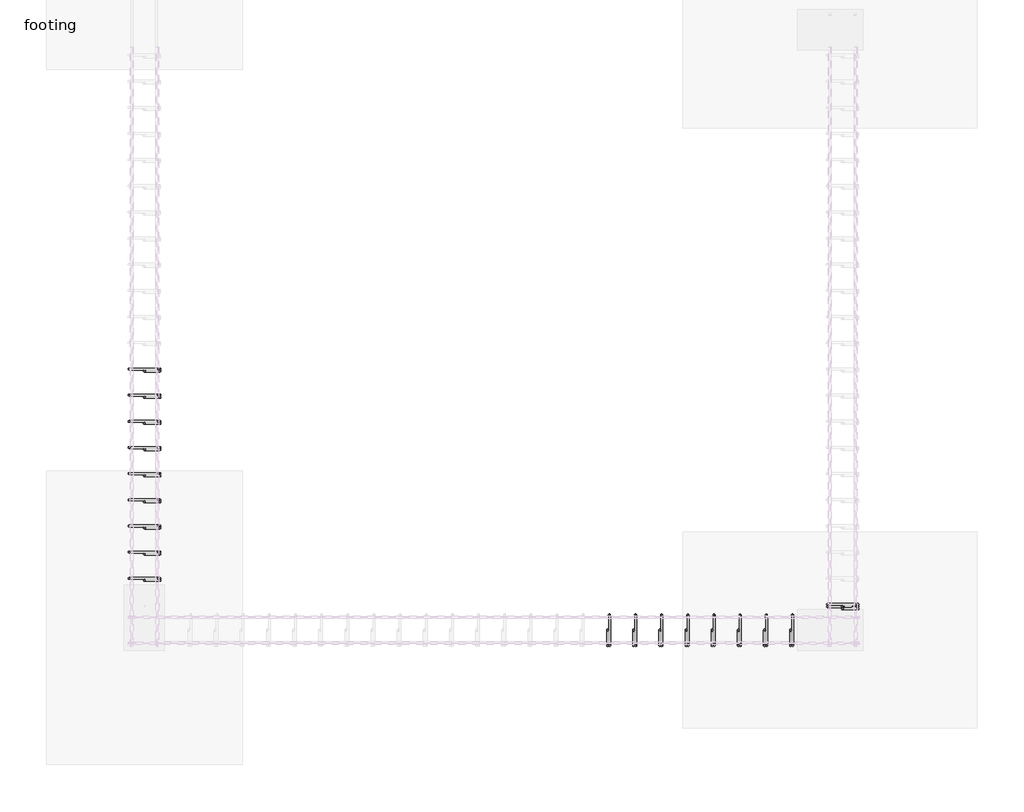
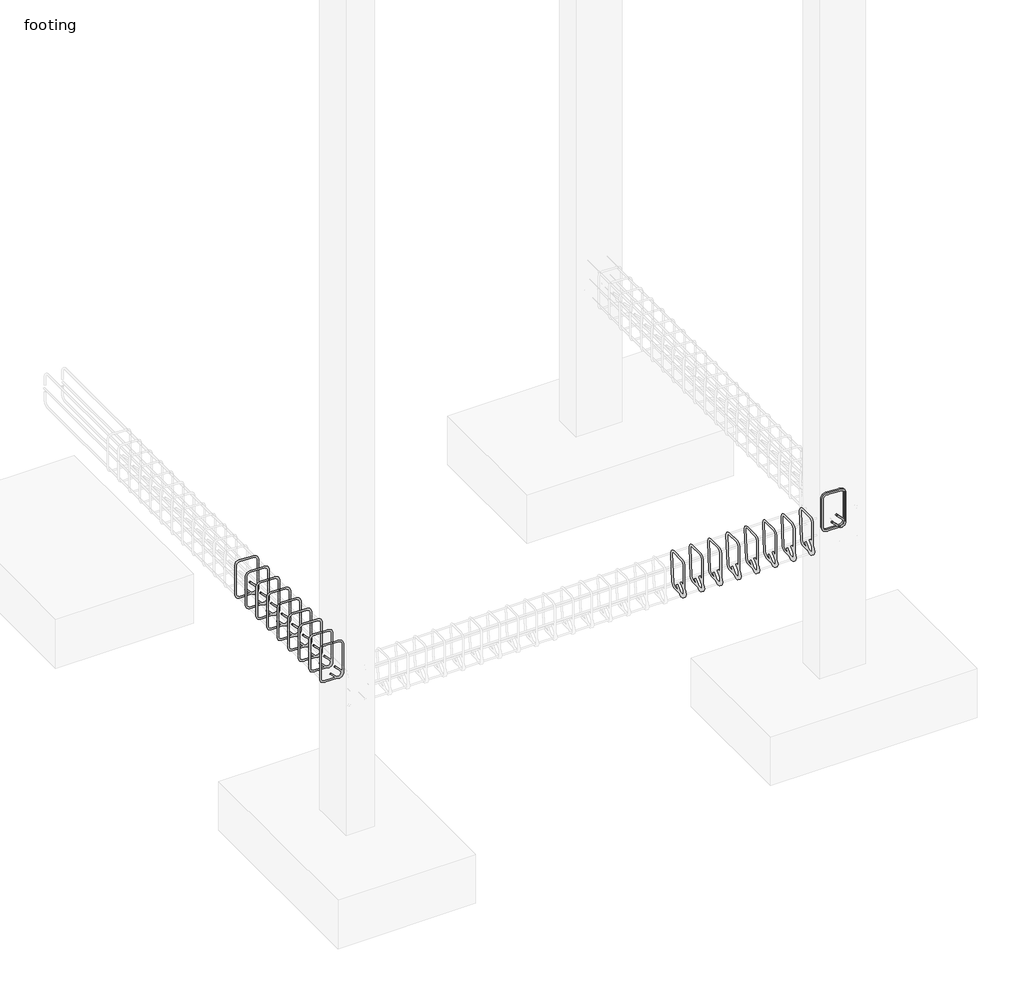
# One storey, part 3 of 21: 19 reinforcing bars.
"""IFC4 building model written with IfcOpenShell, lengths in millimetres."""

from ifc_helpers import new_model, si_unit, point, frame, origin, place, context, project, spatial, polyline, circle_curve, trimmed, segment, composite_curve, element, save
from ifc_brep_helpers import swept_disk

model = new_model("IFC4")

# Units and contexts
model_context = context("Model", 3, world=origin())
ifc_project = project(units=[si_unit("LENGTHUNIT", "METRE", prefix="MILLI")], contexts=[model_context])

# Site, building, storey
site = spatial("IfcSite", under=ifc_project)
building = spatial("IfcBuilding", under=site)
storey = spatial("IfcBuildingStorey", under=building, Name="footing", Elevation=-1524.0)

# Reinforcing bars
placement = place(None, origin())
element("IfcReinforcingBar", 1, at=placement, inside=storey, context=model_context, shape_type="SolidModel", body=[
    swept_disk(composite_curve([segment(polyline([(-9329.0883428, -282.6612868, -310.8825168), (-9329.0883428, -337.5262853, -365.7475153)]), True, "CONTINUOUS"), segment(trimmed(circle_curve(frame((-9329.0883428, -359.9769256, -343.296875), z_axis=(-1.0, 0.0, 0.0), x_axis=(0.0, 22.450640300000032, -22.450640299999975)), 31.75), [point((-9329.0883428, -337.5262853, -365.7475153))], [point((-9329.0883428, -391.7269256, -343.296875))], True, "CARTESIAN"), True, "CONTINUOUS"), segment(polyline([(-9329.0883428, -391.7269256, -343.296875), (-9329.0883428, -391.7269256, -63.103125)]), True, "CONTINUOUS"), segment(trimmed(circle_curve(frame((-9329.0883428, -359.9769256, -63.103125), z_axis=(-1.0, 0.0, 0.0), x_axis=(0.0, -31.75, 0.0)), 31.75), [point((-9329.0883428, -391.7269256, -63.103125))], [point((-9329.0883428, -359.9769256, -31.353125))], True, "CARTESIAN"), True, "CONTINUOUS"), segment(polyline([(-9329.0883428, -359.9769256, -31.353125), (-9329.0883428, -232.1831756, -31.353125)]), True, "CONTINUOUS"), segment(trimmed(circle_curve(frame((-9327.9159328, -232.1831756, -63.0814712), z_axis=(-0.9993179916193466, 0.0, -0.03692629992126919), x_axis=(-1.1724099999992177, 0.0, 31.728346200000004)), 31.75), [point((-9329.0883428, -232.1831756, -31.353125))], [point((-9327.9159328, -200.4331756, -63.0814712))], True, "CARTESIAN"), True, "CONTINUOUS"), segment(polyline([(-9327.9159328, -200.4331756, -63.0814712), (-9317.5607528, -200.4331756, -343.3185288)]), True, "CONTINUOUS"), segment(trimmed(circle_curve(frame((-9317.5607528, -232.1831756, -343.3185288), z_axis=(-0.9993179916193466, 0.0, -0.03692629992126919), x_axis=(0.0, 31.75, 0.0)), 31.75), [point((-9317.5607528, -200.4331756, -343.3185288))], [point((-9316.3883428, -232.1831756, -375.046875))], True, "CARTESIAN"), True, "CONTINUOUS"), segment(polyline([(-9316.3883428, -232.1831756, -375.046875), (-9316.3883428, -359.9769256, -375.046875)]), True, "CONTINUOUS"), segment(trimmed(circle_curve(frame((-9316.3883428, -359.9769256, -343.296875), z_axis=(-1.0, 0.0, 0.0), x_axis=(0.0, 0.0, -31.75)), 31.75), [point((-9316.3883428, -359.9769256, -375.046875))], [point((-9316.3883428, -382.4275659, -320.8462347))], True, "CARTESIAN"), True, "CONTINUOUS"), segment(polyline([(-9316.3883428, -382.4275659, -320.8462347), (-9316.3883428, -327.5625674, -265.9812362)]), True, "CONTINUOUS")], self_intersect=False), 6.35),
])
element("IfcReinforcingBar", 2, at=placement, inside=storey, context=model_context, shape_type="SolidModel", body=[
    swept_disk(composite_curve([segment(polyline([(-9166.3883428, -282.6612868, -310.8825168), (-9166.3883428, -337.5262853, -365.7475153)]), True, "CONTINUOUS"), segment(trimmed(circle_curve(frame((-9166.3883428, -359.9769256, -343.296875), z_axis=(-1.0, 0.0, 0.0), x_axis=(0.0, 22.450640300000032, -22.450640299999975)), 31.75), [point((-9166.3883428, -337.5262853, -365.7475153))], [point((-9166.3883428, -391.7269256, -343.296875))], True, "CARTESIAN"), True, "CONTINUOUS"), segment(polyline([(-9166.3883428, -391.7269256, -343.296875), (-9166.3883428, -391.7269256, -63.103125)]), True, "CONTINUOUS"), segment(trimmed(circle_curve(frame((-9166.3883428, -359.9769256, -63.103125), z_axis=(-1.0, 0.0, 0.0), x_axis=(0.0, -31.75, 0.0)), 31.75), [point((-9166.3883428, -391.7269256, -63.103125))], [point((-9166.3883428, -359.9769256, -31.353125))], True, "CARTESIAN"), True, "CONTINUOUS"), segment(polyline([(-9166.3883428, -359.9769256, -31.353125), (-9166.3883428, -232.1831756, -31.353125)]), True, "CONTINUOUS"), segment(trimmed(circle_curve(frame((-9165.2159328, -232.1831756, -63.0814712), z_axis=(-0.9993179916193466, 0.0, -0.03692629992126919), x_axis=(-1.1724100000010367, 0.0, 31.728346200000004)), 31.75), [point((-9166.3883428, -232.1831756, -31.353125))], [point((-9165.2159328, -200.4331756, -63.0814712))], True, "CARTESIAN"), True, "CONTINUOUS"), segment(polyline([(-9165.2159328, -200.4331756, -63.0814712), (-9154.8607528, -200.4331756, -343.3185288)]), True, "CONTINUOUS"), segment(trimmed(circle_curve(frame((-9154.8607528, -232.1831756, -343.3185288), z_axis=(-0.9993179916193466, 0.0, -0.03692629992126919), x_axis=(0.0, 31.75, 0.0)), 31.75), [point((-9154.8607528, -200.4331756, -343.3185288))], [point((-9153.6883428, -232.1831756, -375.046875))], True, "CARTESIAN"), True, "CONTINUOUS"), segment(polyline([(-9153.6883428, -232.1831756, -375.046875), (-9153.6883428, -359.9769256, -375.046875)]), True, "CONTINUOUS"), segment(trimmed(circle_curve(frame((-9153.6883428, -359.9769256, -343.296875), z_axis=(-1.0, 0.0, 0.0), x_axis=(0.0, 0.0, -31.75)), 31.75), [point((-9153.6883428, -359.9769256, -375.046875))], [point((-9153.6883428, -382.4275659, -320.8462347))], True, "CARTESIAN"), True, "CONTINUOUS"), segment(polyline([(-9153.6883428, -382.4275659, -320.8462347), (-9153.6883428, -327.5625674, -265.9812362)]), True, "CONTINUOUS")], self_intersect=False), 6.35),
])
element("IfcReinforcingBar", 3, at=placement, inside=storey, context=model_context, shape_type="SolidModel", body=[
    swept_disk(composite_curve([segment(polyline([(-9003.6883428, -282.6612868, -310.8825168), (-9003.6883428, -337.5262853, -365.7475153)]), True, "CONTINUOUS"), segment(trimmed(circle_curve(frame((-9003.6883428, -359.9769256, -343.296875), z_axis=(-1.0, 0.0, 0.0), x_axis=(0.0, 22.450640300000032, -22.450640299999975)), 31.75), [point((-9003.6883428, -337.5262853, -365.7475153))], [point((-9003.6883428, -391.7269256, -343.296875))], True, "CARTESIAN"), True, "CONTINUOUS"), segment(polyline([(-9003.6883428, -391.7269256, -343.296875), (-9003.6883428, -391.7269256, -63.103125)]), True, "CONTINUOUS"), segment(trimmed(circle_curve(frame((-9003.6883428, -359.9769256, -63.103125), z_axis=(-1.0, 0.0, 0.0), x_axis=(0.0, -31.75, 0.0)), 31.75), [point((-9003.6883428, -391.7269256, -63.103125))], [point((-9003.6883428, -359.9769256, -31.353125))], True, "CARTESIAN"), True, "CONTINUOUS"), segment(polyline([(-9003.6883428, -359.9769256, -31.353125), (-9003.6883428, -232.1831756, -31.353125)]), True, "CONTINUOUS"), segment(trimmed(circle_curve(frame((-9002.5159328, -232.1831756, -63.0814712), z_axis=(-0.9993179916193466, 0.0, -0.03692629992126919), x_axis=(-1.1724099999992177, 0.0, 31.728346200000004)), 31.75), [point((-9003.6883428, -232.1831756, -31.353125))], [point((-9002.5159328, -200.4331756, -63.0814712))], True, "CARTESIAN"), True, "CONTINUOUS"), segment(polyline([(-9002.5159328, -200.4331756, -63.0814712), (-8992.1607528, -200.4331756, -343.3185288)]), True, "CONTINUOUS"), segment(trimmed(circle_curve(frame((-8992.1607528, -232.1831756, -343.3185288), z_axis=(-0.9993179916193466, 0.0, -0.03692629992126919), x_axis=(0.0, 31.75, 0.0)), 31.75), [point((-8992.1607528, -200.4331756, -343.3185288))], [point((-8990.9883428, -232.1831756, -375.046875))], True, "CARTESIAN"), True, "CONTINUOUS"), segment(polyline([(-8990.9883428, -232.1831756, -375.046875), (-8990.9883428, -359.9769256, -375.046875)]), True, "CONTINUOUS"), segment(trimmed(circle_curve(frame((-8990.9883428, -359.9769256, -343.296875), z_axis=(-1.0, 0.0, 0.0), x_axis=(0.0, 0.0, -31.75)), 31.75), [point((-8990.9883428, -359.9769256, -375.046875))], [point((-8990.9883428, -382.4275659, -320.8462347))], True, "CARTESIAN"), True, "CONTINUOUS"), segment(polyline([(-8990.9883428, -382.4275659, -320.8462347), (-8990.9883428, -327.5625674, -265.9812362)]), True, "CONTINUOUS")], self_intersect=False), 6.35),
])
element("IfcReinforcingBar", 4, at=placement, inside=storey, context=model_context, shape_type="SolidModel", body=[
    swept_disk(composite_curve([segment(polyline([(-8840.9883428, -282.6612868, -310.8825168), (-8840.9883428, -337.5262853, -365.7475153)]), True, "CONTINUOUS"), segment(trimmed(circle_curve(frame((-8840.9883428, -359.9769256, -343.296875), z_axis=(-1.0, 0.0, 0.0), x_axis=(0.0, 22.450640300000032, -22.450640299999975)), 31.75), [point((-8840.9883428, -337.5262853, -365.7475153))], [point((-8840.9883428, -391.7269256, -343.296875))], True, "CARTESIAN"), True, "CONTINUOUS"), segment(polyline([(-8840.9883428, -391.7269256, -343.296875), (-8840.9883428, -391.7269256, -63.103125)]), True, "CONTINUOUS"), segment(trimmed(circle_curve(frame((-8840.9883428, -359.9769256, -63.103125), z_axis=(-1.0, 0.0, 0.0), x_axis=(0.0, -31.75, 0.0)), 31.75), [point((-8840.9883428, -391.7269256, -63.103125))], [point((-8840.9883428, -359.9769256, -31.353125))], True, "CARTESIAN"), True, "CONTINUOUS"), segment(polyline([(-8840.9883428, -359.9769256, -31.353125), (-8840.9883428, -232.1831756, -31.353125)]), True, "CONTINUOUS"), segment(trimmed(circle_curve(frame((-8839.8159328, -232.1831756, -63.0814712), z_axis=(-0.9993179916193466, 0.0, -0.03692629992126919), x_axis=(-1.1724099999992177, 0.0, 31.728346200000004)), 31.75), [point((-8840.9883428, -232.1831756, -31.353125))], [point((-8839.8159328, -200.4331756, -63.0814712))], True, "CARTESIAN"), True, "CONTINUOUS"), segment(polyline([(-8839.8159328, -200.4331756, -63.0814712), (-8829.4607528, -200.4331756, -343.3185288)]), True, "CONTINUOUS"), segment(trimmed(circle_curve(frame((-8829.4607528, -232.1831756, -343.3185288), z_axis=(-0.9993179916193466, 0.0, -0.03692629992126919), x_axis=(0.0, 31.75, 0.0)), 31.75), [point((-8829.4607528, -200.4331756, -343.3185288))], [point((-8828.2883428, -232.1831756, -375.046875))], True, "CARTESIAN"), True, "CONTINUOUS"), segment(polyline([(-8828.2883428, -232.1831756, -375.046875), (-8828.2883428, -359.9769256, -375.046875)]), True, "CONTINUOUS"), segment(trimmed(circle_curve(frame((-8828.2883428, -359.9769256, -343.296875), z_axis=(-1.0, 0.0, 0.0), x_axis=(0.0, 0.0, -31.75)), 31.75), [point((-8828.2883428, -359.9769256, -375.046875))], [point((-8828.2883428, -382.4275659, -320.8462347))], True, "CARTESIAN"), True, "CONTINUOUS"), segment(polyline([(-8828.2883428, -382.4275659, -320.8462347), (-8828.2883428, -327.5625674, -265.9812362)]), True, "CONTINUOUS")], self_intersect=False), 6.35),
])
element("IfcReinforcingBar", 5, at=placement, inside=storey, context=model_context, shape_type="SolidModel", body=[
    swept_disk(composite_curve([segment(polyline([(-8678.2883428, -282.6612868, -310.8825168), (-8678.2883428, -337.5262853, -365.7475153)]), True, "CONTINUOUS"), segment(trimmed(circle_curve(frame((-8678.2883428, -359.9769256, -343.296875), z_axis=(-1.0, 0.0, 0.0), x_axis=(0.0, 22.450640300000032, -22.450640299999975)), 31.75), [point((-8678.2883428, -337.5262853, -365.7475153))], [point((-8678.2883428, -391.7269256, -343.296875))], True, "CARTESIAN"), True, "CONTINUOUS"), segment(polyline([(-8678.2883428, -391.7269256, -343.296875), (-8678.2883428, -391.7269256, -63.103125)]), True, "CONTINUOUS"), segment(trimmed(circle_curve(frame((-8678.2883428, -359.9769256, -63.103125), z_axis=(-1.0, 0.0, 0.0), x_axis=(0.0, -31.75, 0.0)), 31.75), [point((-8678.2883428, -391.7269256, -63.103125))], [point((-8678.2883428, -359.9769256, -31.353125))], True, "CARTESIAN"), True, "CONTINUOUS"), segment(polyline([(-8678.2883428, -359.9769256, -31.353125), (-8678.2883428, -232.1831756, -31.353125)]), True, "CONTINUOUS"), segment(trimmed(circle_curve(frame((-8677.1159328, -232.1831756, -63.0814712), z_axis=(-0.9993179916193466, 0.0, -0.03692629992126919), x_axis=(-1.1724100000010367, 0.0, 31.728346200000004)), 31.75), [point((-8678.2883428, -232.1831756, -31.353125))], [point((-8677.1159328, -200.4331756, -63.0814712))], True, "CARTESIAN"), True, "CONTINUOUS"), segment(polyline([(-8677.1159328, -200.4331756, -63.0814712), (-8666.7607528, -200.4331756, -343.3185288)]), True, "CONTINUOUS"), segment(trimmed(circle_curve(frame((-8666.7607528, -232.1831756, -343.3185288), z_axis=(-0.9993179916193466, 0.0, -0.03692629992126919), x_axis=(0.0, 31.75, 0.0)), 31.75), [point((-8666.7607528, -200.4331756, -343.3185288))], [point((-8665.5883428, -232.1831756, -375.046875))], True, "CARTESIAN"), True, "CONTINUOUS"), segment(polyline([(-8665.5883428, -232.1831756, -375.046875), (-8665.5883428, -359.9769256, -375.046875)]), True, "CONTINUOUS"), segment(trimmed(circle_curve(frame((-8665.5883428, -359.9769256, -343.296875), z_axis=(-1.0, 0.0, 0.0), x_axis=(0.0, 0.0, -31.75)), 31.75), [point((-8665.5883428, -359.9769256, -375.046875))], [point((-8665.5883428, -382.4275659, -320.8462347))], True, "CARTESIAN"), True, "CONTINUOUS"), segment(polyline([(-8665.5883428, -382.4275659, -320.8462347), (-8665.5883428, -327.5625674, -265.9812362)]), True, "CONTINUOUS")], self_intersect=False), 6.35),
])
element("IfcReinforcingBar", 6, at=placement, inside=storey, context=model_context, shape_type="SolidModel", body=[
    swept_disk(composite_curve([segment(polyline([(-8515.5883428, -282.6612868, -310.8825168), (-8515.5883428, -337.5262853, -365.7475153)]), True, "CONTINUOUS"), segment(trimmed(circle_curve(frame((-8515.5883428, -359.9769256, -343.296875), z_axis=(-1.0, 0.0, 0.0), x_axis=(0.0, 22.450640300000032, -22.450640299999975)), 31.75), [point((-8515.5883428, -337.5262853, -365.7475153))], [point((-8515.5883428, -391.7269256, -343.296875))], True, "CARTESIAN"), True, "CONTINUOUS"), segment(polyline([(-8515.5883428, -391.7269256, -343.296875), (-8515.5883428, -391.7269256, -63.103125)]), True, "CONTINUOUS"), segment(trimmed(circle_curve(frame((-8515.5883428, -359.9769256, -63.103125), z_axis=(-1.0, 0.0, 0.0), x_axis=(0.0, -31.75, 0.0)), 31.75), [point((-8515.5883428, -391.7269256, -63.103125))], [point((-8515.5883428, -359.9769256, -31.353125))], True, "CARTESIAN"), True, "CONTINUOUS"), segment(polyline([(-8515.5883428, -359.9769256, -31.353125), (-8515.5883428, -232.1831756, -31.353125)]), True, "CONTINUOUS"), segment(trimmed(circle_curve(frame((-8514.4159328, -232.1831756, -63.0814712), z_axis=(-0.9993179916193466, 0.0, -0.03692629992126919), x_axis=(-1.1724099999992177, 0.0, 31.728346200000004)), 31.75), [point((-8515.5883428, -232.1831756, -31.353125))], [point((-8514.4159328, -200.4331756, -63.0814712))], True, "CARTESIAN"), True, "CONTINUOUS"), segment(polyline([(-8514.4159328, -200.4331756, -63.0814712), (-8504.0607528, -200.4331756, -343.3185288)]), True, "CONTINUOUS"), segment(trimmed(circle_curve(frame((-8504.0607528, -232.1831756, -343.3185288), z_axis=(-0.9993179916193466, 0.0, -0.03692629992126919), x_axis=(0.0, 31.75, 0.0)), 31.75), [point((-8504.0607528, -200.4331756, -343.3185288))], [point((-8502.8883428, -232.1831756, -375.046875))], True, "CARTESIAN"), True, "CONTINUOUS"), segment(polyline([(-8502.8883428, -232.1831756, -375.046875), (-8502.8883428, -359.9769256, -375.046875)]), True, "CONTINUOUS"), segment(trimmed(circle_curve(frame((-8502.8883428, -359.9769256, -343.296875), z_axis=(-1.0, 0.0, 0.0), x_axis=(0.0, 0.0, -31.75)), 31.75), [point((-8502.8883428, -359.9769256, -375.046875))], [point((-8502.8883428, -382.4275659, -320.8462347))], True, "CARTESIAN"), True, "CONTINUOUS"), segment(polyline([(-8502.8883428, -382.4275659, -320.8462347), (-8502.8883428, -327.5625674, -265.9812362)]), True, "CONTINUOUS")], self_intersect=False), 6.35),
])
element("IfcReinforcingBar", 7, at=placement, inside=storey, context=model_context, shape_type="SolidModel", body=[
    swept_disk(composite_curve([segment(polyline([(-8352.8883428, -282.6612868, -310.8825168), (-8352.8883428, -337.5262853, -365.7475153)]), True, "CONTINUOUS"), segment(trimmed(circle_curve(frame((-8352.8883428, -359.9769256, -343.296875), z_axis=(-1.0, 0.0, 0.0), x_axis=(0.0, 22.450640300000032, -22.450640299999975)), 31.75), [point((-8352.8883428, -337.5262853, -365.7475153))], [point((-8352.8883428, -391.7269256, -343.296875))], True, "CARTESIAN"), True, "CONTINUOUS"), segment(polyline([(-8352.8883428, -391.7269256, -343.296875), (-8352.8883428, -391.7269256, -63.103125)]), True, "CONTINUOUS"), segment(trimmed(circle_curve(frame((-8352.8883428, -359.9769256, -63.103125), z_axis=(-1.0, 0.0, 0.0), x_axis=(0.0, -31.75, 0.0)), 31.75), [point((-8352.8883428, -391.7269256, -63.103125))], [point((-8352.8883428, -359.9769256, -31.353125))], True, "CARTESIAN"), True, "CONTINUOUS"), segment(polyline([(-8352.8883428, -359.9769256, -31.353125), (-8352.8883428, -232.1831756, -31.353125)]), True, "CONTINUOUS"), segment(trimmed(circle_curve(frame((-8351.7159328, -232.1831756, -63.0814712), z_axis=(-0.9993179916193466, 0.0, -0.03692629992126919), x_axis=(-1.1724100000010367, 0.0, 31.728346200000004)), 31.75), [point((-8352.8883428, -232.1831756, -31.353125))], [point((-8351.7159328, -200.4331756, -63.0814712))], True, "CARTESIAN"), True, "CONTINUOUS"), segment(polyline([(-8351.7159328, -200.4331756, -63.0814712), (-8341.3607528, -200.4331756, -343.3185288)]), True, "CONTINUOUS"), segment(trimmed(circle_curve(frame((-8341.3607528, -232.1831756, -343.3185288), z_axis=(-0.9993179916193466, 0.0, -0.03692629992126919), x_axis=(0.0, 31.75, 0.0)), 31.75), [point((-8341.3607528, -200.4331756, -343.3185288))], [point((-8340.1883428, -232.1831756, -375.046875))], True, "CARTESIAN"), True, "CONTINUOUS"), segment(polyline([(-8340.1883428, -232.1831756, -375.046875), (-8340.1883428, -359.9769256, -375.046875)]), True, "CONTINUOUS"), segment(trimmed(circle_curve(frame((-8340.1883428, -359.9769256, -343.296875), z_axis=(-1.0, 0.0, 0.0), x_axis=(0.0, 0.0, -31.75)), 31.75), [point((-8340.1883428, -359.9769256, -375.046875))], [point((-8340.1883428, -382.4275659, -320.8462347))], True, "CARTESIAN"), True, "CONTINUOUS"), segment(polyline([(-8340.1883428, -382.4275659, -320.8462347), (-8340.1883428, -327.5625674, -265.9812362)]), True, "CONTINUOUS")], self_intersect=False), 6.35),
])
element("IfcReinforcingBar", 8, at=placement, inside=storey, context=model_context, shape_type="SolidModel", body=[
    swept_disk(composite_curve([segment(polyline([(-8190.1883428, -282.6612868, -310.8825168), (-8190.1883428, -337.5262853, -365.7475153)]), True, "CONTINUOUS"), segment(trimmed(circle_curve(frame((-8190.1883428, -359.9769256, -343.296875), z_axis=(-1.0, 0.0, 0.0), x_axis=(0.0, 22.450640300000032, -22.450640299999975)), 31.75), [point((-8190.1883428, -337.5262853, -365.7475153))], [point((-8190.1883428, -391.7269256, -343.296875))], True, "CARTESIAN"), True, "CONTINUOUS"), segment(polyline([(-8190.1883428, -391.7269256, -343.296875), (-8190.1883428, -391.7269256, -63.103125)]), True, "CONTINUOUS"), segment(trimmed(circle_curve(frame((-8190.1883428, -359.9769256, -63.103125), z_axis=(-1.0, 0.0, 0.0), x_axis=(0.0, -31.75, 0.0)), 31.75), [point((-8190.1883428, -391.7269256, -63.103125))], [point((-8190.1883428, -359.9769256, -31.353125))], True, "CARTESIAN"), True, "CONTINUOUS"), segment(polyline([(-8190.1883428, -359.9769256, -31.353125), (-8190.1883428, -232.1831756, -31.353125)]), True, "CONTINUOUS"), segment(trimmed(circle_curve(frame((-8189.0159328, -232.1831756, -63.0814712), z_axis=(-0.9993179916193466, 0.0, -0.03692629992126919), x_axis=(-1.1724100000001272, 0.0, 31.728346200000004)), 31.75), [point((-8190.1883428, -232.1831756, -31.353125))], [point((-8189.0159328, -200.4331756, -63.0814712))], True, "CARTESIAN"), True, "CONTINUOUS"), segment(polyline([(-8189.0159328, -200.4331756, -63.0814712), (-8178.6607528, -200.4331756, -343.3185288)]), True, "CONTINUOUS"), segment(trimmed(circle_curve(frame((-8178.6607528, -232.1831756, -343.3185288), z_axis=(-0.9993179916193466, 0.0, -0.03692629992126919), x_axis=(0.0, 31.75, 0.0)), 31.75), [point((-8178.6607528, -200.4331756, -343.3185288))], [point((-8177.4883428, -232.1831756, -375.046875))], True, "CARTESIAN"), True, "CONTINUOUS"), segment(polyline([(-8177.4883428, -232.1831756, -375.046875), (-8177.4883428, -359.9769256, -375.046875)]), True, "CONTINUOUS"), segment(trimmed(circle_curve(frame((-8177.4883428, -359.9769256, -343.296875), z_axis=(-1.0, 0.0, 0.0), x_axis=(0.0, 0.0, -31.75)), 31.75), [point((-8177.4883428, -359.9769256, -375.046875))], [point((-8177.4883428, -382.4275659, -320.8462347))], True, "CARTESIAN"), True, "CONTINUOUS"), segment(polyline([(-8177.4883428, -382.4275659, -320.8462347), (-8177.4883428, -327.5625674, -265.9812362)]), True, "CONTINUOUS")], self_intersect=False), 6.35),
])
element("IfcReinforcingBar", 9, at=placement, inside=storey, context=model_context, shape_type="SolidModel", body=[
    swept_disk(composite_curve([segment(polyline([(-7834.7165254, -150.0300506, -265.9812362), (-7779.851527, -150.0300506, -320.8462347)]), True, "CONTINUOUS"), segment(trimmed(circle_curve(frame((-7802.3021673, -150.0300506, -343.296875), z_axis=(0.0, 1.0, 0.0), x_axis=(22.450640300000487, 0.0, 22.450640299999975)), 31.75), [point((-7779.851527, -150.0300506, -320.8462347))], [point((-7802.3021673, -150.0300506, -375.046875))], True, "CARTESIAN"), True, "CONTINUOUS"), segment(polyline([(-7802.3021673, -150.0300506, -375.046875), (-7930.0959173, -150.0300506, -375.046875)]), True, "CONTINUOUS"), segment(trimmed(circle_curve(frame((-7930.0959173, -150.0300506, -343.296875), z_axis=(0.0, 1.0, 0.0), x_axis=(0.0, 0.0, -31.75)), 31.75), [point((-7930.0959173, -150.0300506, -375.046875))], [point((-7961.8459173, -150.0300506, -343.296875))], True, "CARTESIAN"), True, "CONTINUOUS"), segment(polyline([(-7961.8459173, -150.0300506, -343.296875), (-7961.8459173, -150.0300506, -63.103125)]), True, "CONTINUOUS"), segment(trimmed(circle_curve(frame((-7930.165658, -152.1333043, -63.103125), z_axis=(0.0662442117686417, 0.9978034397651431, 0.0), x_axis=(-31.680259300000216, 2.103253699999982, 0.0)), 31.75), [point((-7961.8459173, -150.0300506, -63.103125))], [point((-7930.165658, -152.1333043, -31.353125))], True, "CARTESIAN"), True, "CONTINUOUS"), segment(polyline([(-7930.165658, -152.1333043, -31.353125), (-7802.2324265, -160.6267969, -31.353125)]), True, "CONTINUOUS"), segment(trimmed(circle_curve(frame((-7802.2324265, -160.6267969, -63.103125), z_axis=(0.06624421176864169, 0.997803439765143, 0.0), x_axis=(0.0, 0.0, 31.75)), 31.75), [point((-7802.2324265, -160.6267969, -31.353125))], [point((-7770.5521673, -162.7300506, -63.103125))], True, "CARTESIAN"), True, "CONTINUOUS"), segment(polyline([(-7770.5521673, -162.7300506, -63.103125), (-7770.5521673, -162.7300506, -343.296875)]), True, "CONTINUOUS"), segment(trimmed(circle_curve(frame((-7802.3021673, -162.7300506, -343.296875), z_axis=(0.0, 1.0, 0.0), x_axis=(31.75, 0.0, 0.0)), 31.75), [point((-7770.5521673, -162.7300506, -343.296875))], [point((-7824.7528076, -162.7300506, -365.7475153))], True, "CARTESIAN"), True, "CONTINUOUS"), segment(polyline([(-7824.7528076, -162.7300506, -365.7475153), (-7879.617806, -162.7300506, -310.8825168)]), True, "CONTINUOUS")], self_intersect=False), 6.35),
])
element("IfcReinforcingBar", 10, at=placement, inside=storey, context=model_context, shape_type="SolidModel", body=[
    swept_disk(composite_curve([segment(polyline([(-7834.7165254, -135.8043927, -265.9812362), (-7779.851527, -135.8043927, -320.8462347)]), True, "CONTINUOUS"), segment(trimmed(circle_curve(frame((-7802.3021673, -135.8043927, -343.296875), z_axis=(0.0, 1.0, 0.0), x_axis=(22.450640300000487, 0.0, 22.450640299999975)), 31.75), [point((-7779.851527, -135.8043927, -320.8462347))], [point((-7802.3021673, -135.8043927, -375.046875))], True, "CARTESIAN"), True, "CONTINUOUS"), segment(polyline([(-7802.3021673, -135.8043927, -375.046875), (-7930.0959173, -135.8043927, -375.046875)]), True, "CONTINUOUS"), segment(trimmed(circle_curve(frame((-7930.0959173, -135.8043927, -343.296875), z_axis=(0.0, 1.0, 0.0), x_axis=(0.0, 0.0, -31.75)), 31.75), [point((-7930.0959173, -135.8043927, -375.046875))], [point((-7961.8459173, -135.8043927, -343.296875))], True, "CARTESIAN"), True, "CONTINUOUS"), segment(polyline([(-7961.8459173, -135.8043927, -343.296875), (-7961.8459173, -135.8043927, -63.103125)]), True, "CONTINUOUS"), segment(trimmed(circle_curve(frame((-7930.165658, -137.9076464, -63.103125), z_axis=(0.0662442117686417, 0.9978034397651431, 0.0), x_axis=(-31.680259300000216, 2.1032537000000104, 0.0)), 31.75), [point((-7961.8459173, -135.8043927, -63.103125))], [point((-7930.165658, -137.9076464, -31.353125))], True, "CARTESIAN"), True, "CONTINUOUS"), segment(polyline([(-7930.165658, -137.9076464, -31.353125), (-7802.2324265, -146.401139, -31.353125)]), True, "CONTINUOUS"), segment(trimmed(circle_curve(frame((-7802.2324265, -146.401139, -63.103125), z_axis=(0.06624421176864169, 0.997803439765143, 0.0), x_axis=(0.0, 0.0, 31.75)), 31.75), [point((-7802.2324265, -146.401139, -31.353125))], [point((-7770.5521673, -148.5043927, -63.103125))], True, "CARTESIAN"), True, "CONTINUOUS"), segment(polyline([(-7770.5521673, -148.5043927, -63.103125), (-7770.5521673, -148.5043927, -343.296875)]), True, "CONTINUOUS"), segment(trimmed(circle_curve(frame((-7802.3021673, -148.5043927, -343.296875), z_axis=(0.0, 1.0, 0.0), x_axis=(31.75, 0.0, 0.0)), 31.75), [point((-7770.5521673, -148.5043927, -343.296875))], [point((-7824.7528076, -148.5043927, -365.7475153))], True, "CARTESIAN"), True, "CONTINUOUS"), segment(polyline([(-7824.7528076, -148.5043927, -365.7475153), (-7879.617806, -148.5043927, -310.8825168)]), True, "CONTINUOUS")], self_intersect=False), 6.35),
])
element("IfcReinforcingBar", 11, at=placement, inside=storey, context=model_context, shape_type="SolidModel", body=[
    swept_disk(composite_curve([segment(polyline([(-12178.1165254, 26.8956073, -265.9812362), (-12123.251527, 26.8956073, -320.8462347)]), True, "CONTINUOUS"), segment(trimmed(circle_curve(frame((-12145.7021673, 26.8956073, -343.296875), z_axis=(0.0, 1.0, 0.0), x_axis=(22.450640299999577, 0.0, 22.450640299999975)), 31.75), [point((-12123.251527, 26.8956073, -320.8462347))], [point((-12145.7021673, 26.8956073, -375.046875))], True, "CARTESIAN"), True, "CONTINUOUS"), segment(polyline([(-12145.7021673, 26.8956073, -375.046875), (-12273.4959173, 26.8956073, -375.046875)]), True, "CONTINUOUS"), segment(trimmed(circle_curve(frame((-12273.4959173, 26.8956073, -343.296875), z_axis=(0.0, 1.0, 0.0), x_axis=(0.0, 0.0, -31.75)), 31.75), [point((-12273.4959173, 26.8956073, -375.046875))], [point((-12305.2459173, 26.8956073, -343.296875))], True, "CARTESIAN"), True, "CONTINUOUS"), segment(polyline([(-12305.2459173, 26.8956073, -343.296875), (-12305.2459173, 26.8956073, -63.103125)]), True, "CONTINUOUS"), segment(trimmed(circle_curve(frame((-12273.565658, 24.7923536, -63.103125), z_axis=(0.0662442117686417, 0.9978034397651431, 0.0), x_axis=(-31.680259300001126, 2.1032537000000033, 0.0)), 31.75), [point((-12305.2459173, 26.8956073, -63.103125))], [point((-12273.565658, 24.7923536, -31.353125))], True, "CARTESIAN"), True, "CONTINUOUS"), segment(polyline([(-12273.565658, 24.7923536, -31.353125), (-12145.6324265, 16.298861, -31.353125)]), True, "CONTINUOUS"), segment(trimmed(circle_curve(frame((-12145.6324265, 16.298861, -63.103125), z_axis=(0.06624421176864169, 0.997803439765143, 0.0), x_axis=(0.0, 0.0, 31.75)), 31.75), [point((-12145.6324265, 16.298861, -31.353125))], [point((-12113.9521673, 14.1956073, -63.103125))], True, "CARTESIAN"), True, "CONTINUOUS"), segment(polyline([(-12113.9521673, 14.1956073, -63.103125), (-12113.9521673, 14.1956073, -343.296875)]), True, "CONTINUOUS"), segment(trimmed(circle_curve(frame((-12145.7021673, 14.1956073, -343.296875), z_axis=(0.0, 1.0, 0.0), x_axis=(31.75, 0.0, 0.0)), 31.75), [point((-12113.9521673, 14.1956073, -343.296875))], [point((-12168.1528076, 14.1956073, -365.7475153))], True, "CARTESIAN"), True, "CONTINUOUS"), segment(polyline([(-12168.1528076, 14.1956073, -365.7475153), (-12223.017806, 14.1956073, -310.8825168)]), True, "CONTINUOUS")], self_intersect=False), 6.35),
])
element("IfcReinforcingBar", 12, at=placement, inside=storey, context=model_context, shape_type="SolidModel", body=[
    swept_disk(composite_curve([segment(polyline([(-12178.1165254, 189.5956073, -265.9812362), (-12123.251527, 189.5956073, -320.8462347)]), True, "CONTINUOUS"), segment(trimmed(circle_curve(frame((-12145.7021673, 189.5956073, -343.296875), z_axis=(0.0, 1.0, 0.0), x_axis=(22.450640299999577, 0.0, 22.450640299999975)), 31.75), [point((-12123.251527, 189.5956073, -320.8462347))], [point((-12145.7021673, 189.5956073, -375.046875))], True, "CARTESIAN"), True, "CONTINUOUS"), segment(polyline([(-12145.7021673, 189.5956073, -375.046875), (-12273.4959173, 189.5956073, -375.046875)]), True, "CONTINUOUS"), segment(trimmed(circle_curve(frame((-12273.4959173, 189.5956073, -343.296875), z_axis=(0.0, 1.0, 0.0), x_axis=(0.0, 0.0, -31.75)), 31.75), [point((-12273.4959173, 189.5956073, -375.046875))], [point((-12305.2459173, 189.5956073, -343.296875))], True, "CARTESIAN"), True, "CONTINUOUS"), segment(polyline([(-12305.2459173, 189.5956073, -343.296875), (-12305.2459173, 189.5956073, -63.103125)]), True, "CONTINUOUS"), segment(trimmed(circle_curve(frame((-12273.565658, 187.4923536, -63.103125), z_axis=(0.0662442117686417, 0.9978034397651431, 0.0), x_axis=(-31.680259300001126, 2.1032537000000104, 0.0)), 31.75), [point((-12305.2459173, 189.5956073, -63.103125))], [point((-12273.565658, 187.4923536, -31.353125))], True, "CARTESIAN"), True, "CONTINUOUS"), segment(polyline([(-12273.565658, 187.4923536, -31.353125), (-12145.6324265, 178.998861, -31.353125)]), True, "CONTINUOUS"), segment(trimmed(circle_curve(frame((-12145.6324265, 178.998861, -63.103125), z_axis=(0.06624421176864169, 0.997803439765143, 0.0), x_axis=(0.0, 0.0, 31.75)), 31.75), [point((-12145.6324265, 178.998861, -31.353125))], [point((-12113.9521673, 176.8956073, -63.103125))], True, "CARTESIAN"), True, "CONTINUOUS"), segment(polyline([(-12113.9521673, 176.8956073, -63.103125), (-12113.9521673, 176.8956073, -343.296875)]), True, "CONTINUOUS"), segment(trimmed(circle_curve(frame((-12145.7021673, 176.8956073, -343.296875), z_axis=(0.0, 1.0, 0.0), x_axis=(31.75, 0.0, 0.0)), 31.75), [point((-12113.9521673, 176.8956073, -343.296875))], [point((-12168.1528076, 176.8956073, -365.7475153))], True, "CARTESIAN"), True, "CONTINUOUS"), segment(polyline([(-12168.1528076, 176.8956073, -365.7475153), (-12223.017806, 176.8956073, -310.8825168)]), True, "CONTINUOUS")], self_intersect=False), 6.35),
])
element("IfcReinforcingBar", 13, at=placement, inside=storey, context=model_context, shape_type="SolidModel", body=[
    swept_disk(composite_curve([segment(polyline([(-12178.1165254, 352.2956073, -265.9812362), (-12123.251527, 352.2956073, -320.8462347)]), True, "CONTINUOUS"), segment(trimmed(circle_curve(frame((-12145.7021673, 352.2956073, -343.296875), z_axis=(0.0, 1.0, 0.0), x_axis=(22.450640299999577, 0.0, 22.450640299999975)), 31.75), [point((-12123.251527, 352.2956073, -320.8462347))], [point((-12145.7021673, 352.2956073, -375.046875))], True, "CARTESIAN"), True, "CONTINUOUS"), segment(polyline([(-12145.7021673, 352.2956073, -375.046875), (-12273.4959173, 352.2956073, -375.046875)]), True, "CONTINUOUS"), segment(trimmed(circle_curve(frame((-12273.4959173, 352.2956073, -343.296875), z_axis=(0.0, 1.0, 0.0), x_axis=(0.0, 0.0, -31.75)), 31.75), [point((-12273.4959173, 352.2956073, -375.046875))], [point((-12305.2459173, 352.2956073, -343.296875))], True, "CARTESIAN"), True, "CONTINUOUS"), segment(polyline([(-12305.2459173, 352.2956073, -343.296875), (-12305.2459173, 352.2956073, -63.103125)]), True, "CONTINUOUS"), segment(trimmed(circle_curve(frame((-12273.565658, 350.1923536, -63.103125), z_axis=(0.0662442117686417, 0.9978034397651431, 0.0), x_axis=(-31.680259300001126, 2.103253699999982, 0.0)), 31.75), [point((-12305.2459173, 352.2956073, -63.103125))], [point((-12273.565658, 350.1923536, -31.353125))], True, "CARTESIAN"), True, "CONTINUOUS"), segment(polyline([(-12273.565658, 350.1923536, -31.353125), (-12145.6324265, 341.698861, -31.353125)]), True, "CONTINUOUS"), segment(trimmed(circle_curve(frame((-12145.6324265, 341.698861, -63.103125), z_axis=(0.06624421176864169, 0.997803439765143, 0.0), x_axis=(0.0, 0.0, 31.75)), 31.75), [point((-12145.6324265, 341.698861, -31.353125))], [point((-12113.9521673, 339.5956073, -63.103125))], True, "CARTESIAN"), True, "CONTINUOUS"), segment(polyline([(-12113.9521673, 339.5956073, -63.103125), (-12113.9521673, 339.5956073, -343.296875)]), True, "CONTINUOUS"), segment(trimmed(circle_curve(frame((-12145.7021673, 339.5956073, -343.296875), z_axis=(0.0, 1.0, 0.0), x_axis=(31.75, 0.0, 0.0)), 31.75), [point((-12113.9521673, 339.5956073, -343.296875))], [point((-12168.1528076, 339.5956073, -365.7475153))], True, "CARTESIAN"), True, "CONTINUOUS"), segment(polyline([(-12168.1528076, 339.5956073, -365.7475153), (-12223.017806, 339.5956073, -310.8825168)]), True, "CONTINUOUS")], self_intersect=False), 6.35),
])
element("IfcReinforcingBar", 14, at=placement, inside=storey, context=model_context, shape_type="SolidModel", body=[
    swept_disk(composite_curve([segment(polyline([(-12178.1165254, 514.9956073, -265.9812362), (-12123.251527, 514.9956073, -320.8462347)]), True, "CONTINUOUS"), segment(trimmed(circle_curve(frame((-12145.7021673, 514.9956073, -343.296875), z_axis=(0.0, 1.0, 0.0), x_axis=(22.450640299999577, 0.0, 22.450640299999975)), 31.75), [point((-12123.251527, 514.9956073, -320.8462347))], [point((-12145.7021673, 514.9956073, -375.046875))], True, "CARTESIAN"), True, "CONTINUOUS"), segment(polyline([(-12145.7021673, 514.9956073, -375.046875), (-12273.4959173, 514.9956073, -375.046875)]), True, "CONTINUOUS"), segment(trimmed(circle_curve(frame((-12273.4959173, 514.9956073, -343.296875), z_axis=(0.0, 1.0, 0.0), x_axis=(0.0, 0.0, -31.75)), 31.75), [point((-12273.4959173, 514.9956073, -375.046875))], [point((-12305.2459173, 514.9956073, -343.296875))], True, "CARTESIAN"), True, "CONTINUOUS"), segment(polyline([(-12305.2459173, 514.9956073, -343.296875), (-12305.2459173, 514.9956073, -63.103125)]), True, "CONTINUOUS"), segment(trimmed(circle_curve(frame((-12273.565658, 512.8923536, -63.103125), z_axis=(0.0662442117686417, 0.9978034397651431, 0.0), x_axis=(-31.680259300001126, 2.103253699999982, 0.0)), 31.75), [point((-12305.2459173, 514.9956073, -63.103125))], [point((-12273.565658, 512.8923536, -31.353125))], True, "CARTESIAN"), True, "CONTINUOUS"), segment(polyline([(-12273.565658, 512.8923536, -31.353125), (-12145.6324265, 504.398861, -31.353125)]), True, "CONTINUOUS"), segment(trimmed(circle_curve(frame((-12145.6324265, 504.398861, -63.103125), z_axis=(0.06624421176864169, 0.997803439765143, 0.0), x_axis=(0.0, 0.0, 31.75)), 31.75), [point((-12145.6324265, 504.398861, -31.353125))], [point((-12113.9521673, 502.2956073, -63.103125))], True, "CARTESIAN"), True, "CONTINUOUS"), segment(polyline([(-12113.9521673, 502.2956073, -63.103125), (-12113.9521673, 502.2956073, -343.296875)]), True, "CONTINUOUS"), segment(trimmed(circle_curve(frame((-12145.7021673, 502.2956073, -343.296875), z_axis=(0.0, 1.0, 0.0), x_axis=(31.75, 0.0, 0.0)), 31.75), [point((-12113.9521673, 502.2956073, -343.296875))], [point((-12168.1528076, 502.2956073, -365.7475153))], True, "CARTESIAN"), True, "CONTINUOUS"), segment(polyline([(-12168.1528076, 502.2956073, -365.7475153), (-12223.017806, 502.2956073, -310.8825168)]), True, "CONTINUOUS")], self_intersect=False), 6.35),
])
element("IfcReinforcingBar", 15, at=placement, inside=storey, context=model_context, shape_type="SolidModel", body=[
    swept_disk(composite_curve([segment(polyline([(-12178.1165254, 677.6956073, -265.9812362), (-12123.251527, 677.6956073, -320.8462347)]), True, "CONTINUOUS"), segment(trimmed(circle_curve(frame((-12145.7021673, 677.6956073, -343.296875), z_axis=(0.0, 1.0, 0.0), x_axis=(22.450640299999577, 0.0, 22.450640299999975)), 31.75), [point((-12123.251527, 677.6956073, -320.8462347))], [point((-12145.7021673, 677.6956073, -375.046875))], True, "CARTESIAN"), True, "CONTINUOUS"), segment(polyline([(-12145.7021673, 677.6956073, -375.046875), (-12273.4959173, 677.6956073, -375.046875)]), True, "CONTINUOUS"), segment(trimmed(circle_curve(frame((-12273.4959173, 677.6956073, -343.296875), z_axis=(0.0, 1.0, 0.0), x_axis=(0.0, 0.0, -31.75)), 31.75), [point((-12273.4959173, 677.6956073, -375.046875))], [point((-12305.2459173, 677.6956073, -343.296875))], True, "CARTESIAN"), True, "CONTINUOUS"), segment(polyline([(-12305.2459173, 677.6956073, -343.296875), (-12305.2459173, 677.6956073, -63.103125)]), True, "CONTINUOUS"), segment(trimmed(circle_curve(frame((-12273.565658, 675.5923536, -63.103125), z_axis=(0.0662442117686417, 0.9978034397651431, 0.0), x_axis=(-31.680259300001126, 2.103253699999982, 0.0)), 31.75), [point((-12305.2459173, 677.6956073, -63.103125))], [point((-12273.565658, 675.5923536, -31.353125))], True, "CARTESIAN"), True, "CONTINUOUS"), segment(polyline([(-12273.565658, 675.5923536, -31.353125), (-12145.6324265, 667.098861, -31.353125)]), True, "CONTINUOUS"), segment(trimmed(circle_curve(frame((-12145.6324265, 667.098861, -63.103125), z_axis=(0.06624421176864169, 0.997803439765143, 0.0), x_axis=(0.0, 0.0, 31.75)), 31.75), [point((-12145.6324265, 667.098861, -31.353125))], [point((-12113.9521673, 664.9956073, -63.103125))], True, "CARTESIAN"), True, "CONTINUOUS"), segment(polyline([(-12113.9521673, 664.9956073, -63.103125), (-12113.9521673, 664.9956073, -343.296875)]), True, "CONTINUOUS"), segment(trimmed(circle_curve(frame((-12145.7021673, 664.9956073, -343.296875), z_axis=(0.0, 1.0, 0.0), x_axis=(31.75, 0.0, 0.0)), 31.75), [point((-12113.9521673, 664.9956073, -343.296875))], [point((-12168.1528076, 664.9956073, -365.7475153))], True, "CARTESIAN"), True, "CONTINUOUS"), segment(polyline([(-12168.1528076, 664.9956073, -365.7475153), (-12223.017806, 664.9956073, -310.8825168)]), True, "CONTINUOUS")], self_intersect=False), 6.35),
])
element("IfcReinforcingBar", 16, at=placement, inside=storey, context=model_context, shape_type="SolidModel", body=[
    swept_disk(composite_curve([segment(polyline([(-12178.1165254, 840.3956073, -265.9812362), (-12123.251527, 840.3956073, -320.8462347)]), True, "CONTINUOUS"), segment(trimmed(circle_curve(frame((-12145.7021673, 840.3956073, -343.296875), z_axis=(0.0, 1.0, 0.0), x_axis=(22.450640299999577, 0.0, 22.450640299999975)), 31.75), [point((-12123.251527, 840.3956073, -320.8462347))], [point((-12145.7021673, 840.3956073, -375.046875))], True, "CARTESIAN"), True, "CONTINUOUS"), segment(polyline([(-12145.7021673, 840.3956073, -375.046875), (-12273.4959173, 840.3956073, -375.046875)]), True, "CONTINUOUS"), segment(trimmed(circle_curve(frame((-12273.4959173, 840.3956073, -343.296875), z_axis=(0.0, 1.0, 0.0), x_axis=(0.0, 0.0, -31.75)), 31.75), [point((-12273.4959173, 840.3956073, -375.046875))], [point((-12305.2459173, 840.3956073, -343.296875))], True, "CARTESIAN"), True, "CONTINUOUS"), segment(polyline([(-12305.2459173, 840.3956073, -343.296875), (-12305.2459173, 840.3956073, -63.103125)]), True, "CONTINUOUS"), segment(trimmed(circle_curve(frame((-12273.565658, 838.2923536, -63.103125), z_axis=(0.0662442117686417, 0.9978034397651431, 0.0), x_axis=(-31.680259300001126, 2.1032537000000957, 0.0)), 31.75), [point((-12305.2459173, 840.3956073, -63.103125))], [point((-12273.565658, 838.2923536, -31.353125))], True, "CARTESIAN"), True, "CONTINUOUS"), segment(polyline([(-12273.565658, 838.2923536, -31.353125), (-12145.6324265, 829.798861, -31.353125)]), True, "CONTINUOUS"), segment(trimmed(circle_curve(frame((-12145.6324265, 829.798861, -63.103125), z_axis=(0.06624421176864169, 0.997803439765143, 0.0), x_axis=(0.0, 0.0, 31.75)), 31.75), [point((-12145.6324265, 829.798861, -31.353125))], [point((-12113.9521673, 827.6956073, -63.103125))], True, "CARTESIAN"), True, "CONTINUOUS"), segment(polyline([(-12113.9521673, 827.6956073, -63.103125), (-12113.9521673, 827.6956073, -343.296875)]), True, "CONTINUOUS"), segment(trimmed(circle_curve(frame((-12145.7021673, 827.6956073, -343.296875), z_axis=(0.0, 1.0, 0.0), x_axis=(31.75, 0.0, 0.0)), 31.75), [point((-12113.9521673, 827.6956073, -343.296875))], [point((-12168.1528076, 827.6956073, -365.7475153))], True, "CARTESIAN"), True, "CONTINUOUS"), segment(polyline([(-12168.1528076, 827.6956073, -365.7475153), (-12223.017806, 827.6956073, -310.8825168)]), True, "CONTINUOUS")], self_intersect=False), 6.35),
])
element("IfcReinforcingBar", 17, at=placement, inside=storey, context=model_context, shape_type="SolidModel", body=[
    swept_disk(composite_curve([segment(polyline([(-12178.1165254, 1003.0956073, -265.9812362), (-12123.251527, 1003.0956073, -320.8462347)]), True, "CONTINUOUS"), segment(trimmed(circle_curve(frame((-12145.7021673, 1003.0956073, -343.296875), z_axis=(0.0, 1.0, 0.0), x_axis=(22.450640299999577, 0.0, 22.450640299999975)), 31.75), [point((-12123.251527, 1003.0956073, -320.8462347))], [point((-12145.7021673, 1003.0956073, -375.046875))], True, "CARTESIAN"), True, "CONTINUOUS"), segment(polyline([(-12145.7021673, 1003.0956073, -375.046875), (-12273.4959173, 1003.0956073, -375.046875)]), True, "CONTINUOUS"), segment(trimmed(circle_curve(frame((-12273.4959173, 1003.0956073, -343.296875), z_axis=(0.0, 1.0, 0.0), x_axis=(0.0, 0.0, -31.75)), 31.75), [point((-12273.4959173, 1003.0956073, -375.046875))], [point((-12305.2459173, 1003.0956073, -343.296875))], True, "CARTESIAN"), True, "CONTINUOUS"), segment(polyline([(-12305.2459173, 1003.0956073, -343.296875), (-12305.2459173, 1003.0956073, -63.103125)]), True, "CONTINUOUS"), segment(trimmed(circle_curve(frame((-12273.565658, 1000.9923536, -63.103125), z_axis=(0.0662442117686417, 0.9978034397651431, 0.0), x_axis=(-31.680259300001126, 2.103253699999982, 0.0)), 31.75), [point((-12305.2459173, 1003.0956073, -63.103125))], [point((-12273.565658, 1000.9923536, -31.353125))], True, "CARTESIAN"), True, "CONTINUOUS"), segment(polyline([(-12273.565658, 1000.9923536, -31.353125), (-12145.6324265, 992.498861, -31.353125)]), True, "CONTINUOUS"), segment(trimmed(circle_curve(frame((-12145.6324265, 992.498861, -63.103125), z_axis=(0.06624421176864169, 0.997803439765143, 0.0), x_axis=(0.0, 0.0, 31.75)), 31.75), [point((-12145.6324265, 992.498861, -31.353125))], [point((-12113.9521673, 990.3956073, -63.103125))], True, "CARTESIAN"), True, "CONTINUOUS"), segment(polyline([(-12113.9521673, 990.3956073, -63.103125), (-12113.9521673, 990.3956073, -343.296875)]), True, "CONTINUOUS"), segment(trimmed(circle_curve(frame((-12145.7021673, 990.3956073, -343.296875), z_axis=(0.0, 1.0, 0.0), x_axis=(31.75, 0.0, 0.0)), 31.75), [point((-12113.9521673, 990.3956073, -343.296875))], [point((-12168.1528076, 990.3956073, -365.7475153))], True, "CARTESIAN"), True, "CONTINUOUS"), segment(polyline([(-12168.1528076, 990.3956073, -365.7475153), (-12223.017806, 990.3956073, -310.8825168)]), True, "CONTINUOUS")], self_intersect=False), 6.35),
])
element("IfcReinforcingBar", 18, at=placement, inside=storey, context=model_context, shape_type="SolidModel", body=[
    swept_disk(composite_curve([segment(polyline([(-12178.1165254, 1165.7956073, -265.9812362), (-12123.251527, 1165.7956073, -320.8462347)]), True, "CONTINUOUS"), segment(trimmed(circle_curve(frame((-12145.7021673, 1165.7956073, -343.296875), z_axis=(0.0, 1.0, 0.0), x_axis=(22.450640299999577, 0.0, 22.450640299999975)), 31.75), [point((-12123.251527, 1165.7956073, -320.8462347))], [point((-12145.7021673, 1165.7956073, -375.046875))], True, "CARTESIAN"), True, "CONTINUOUS"), segment(polyline([(-12145.7021673, 1165.7956073, -375.046875), (-12273.4959173, 1165.7956073, -375.046875)]), True, "CONTINUOUS"), segment(trimmed(circle_curve(frame((-12273.4959173, 1165.7956073, -343.296875), z_axis=(0.0, 1.0, 0.0), x_axis=(0.0, 0.0, -31.75)), 31.75), [point((-12273.4959173, 1165.7956073, -375.046875))], [point((-12305.2459173, 1165.7956073, -343.296875))], True, "CARTESIAN"), True, "CONTINUOUS"), segment(polyline([(-12305.2459173, 1165.7956073, -343.296875), (-12305.2459173, 1165.7956073, -63.103125)]), True, "CONTINUOUS"), segment(trimmed(circle_curve(frame((-12273.565658, 1163.6923536, -63.103125), z_axis=(0.0662442117686417, 0.9978034397651431, 0.0), x_axis=(-31.680259300001126, 2.1032537000000957, 0.0)), 31.75), [point((-12305.2459173, 1165.7956073, -63.103125))], [point((-12273.565658, 1163.6923536, -31.353125))], True, "CARTESIAN"), True, "CONTINUOUS"), segment(polyline([(-12273.565658, 1163.6923536, -31.353125), (-12145.6324265, 1155.198861, -31.353125)]), True, "CONTINUOUS"), segment(trimmed(circle_curve(frame((-12145.6324265, 1155.198861, -63.103125), z_axis=(0.06624421176864169, 0.997803439765143, 0.0), x_axis=(0.0, 0.0, 31.75)), 31.75), [point((-12145.6324265, 1155.198861, -31.353125))], [point((-12113.9521673, 1153.0956073, -63.103125))], True, "CARTESIAN"), True, "CONTINUOUS"), segment(polyline([(-12113.9521673, 1153.0956073, -63.103125), (-12113.9521673, 1153.0956073, -343.296875)]), True, "CONTINUOUS"), segment(trimmed(circle_curve(frame((-12145.7021673, 1153.0956073, -343.296875), z_axis=(0.0, 1.0, 0.0), x_axis=(31.75, 0.0, 0.0)), 31.75), [point((-12113.9521673, 1153.0956073, -343.296875))], [point((-12168.1528076, 1153.0956073, -365.7475153))], True, "CARTESIAN"), True, "CONTINUOUS"), segment(polyline([(-12168.1528076, 1153.0956073, -365.7475153), (-12223.017806, 1153.0956073, -310.8825168)]), True, "CONTINUOUS")], self_intersect=False), 6.35),
])
element("IfcReinforcingBar", 19, at=placement, inside=storey, context=model_context, shape_type="SolidModel", body=[
    swept_disk(composite_curve([segment(polyline([(-12178.1165254, 1328.4956073, -265.9812362), (-12123.251527, 1328.4956073, -320.8462347)]), True, "CONTINUOUS"), segment(trimmed(circle_curve(frame((-12145.7021673, 1328.4956073, -343.296875), z_axis=(0.0, 1.0, 0.0), x_axis=(22.450640299999577, 0.0, 22.450640299999975)), 31.75), [point((-12123.251527, 1328.4956073, -320.8462347))], [point((-12145.7021673, 1328.4956073, -375.046875))], True, "CARTESIAN"), True, "CONTINUOUS"), segment(polyline([(-12145.7021673, 1328.4956073, -375.046875), (-12273.4959173, 1328.4956073, -375.046875)]), True, "CONTINUOUS"), segment(trimmed(circle_curve(frame((-12273.4959173, 1328.4956073, -343.296875), z_axis=(0.0, 1.0, 0.0), x_axis=(0.0, 0.0, -31.75)), 31.75), [point((-12273.4959173, 1328.4956073, -375.046875))], [point((-12305.2459173, 1328.4956073, -343.296875))], True, "CARTESIAN"), True, "CONTINUOUS"), segment(polyline([(-12305.2459173, 1328.4956073, -343.296875), (-12305.2459173, 1328.4956073, -63.103125)]), True, "CONTINUOUS"), segment(trimmed(circle_curve(frame((-12273.565658, 1326.3923536, -63.103125), z_axis=(0.0662442117686417, 0.9978034397651431, 0.0), x_axis=(-31.680259300001126, 2.1032537000000957, 0.0)), 31.75), [point((-12305.2459173, 1328.4956073, -63.103125))], [point((-12273.565658, 1326.3923536, -31.353125))], True, "CARTESIAN"), True, "CONTINUOUS"), segment(polyline([(-12273.565658, 1326.3923536, -31.353125), (-12145.6324265, 1317.898861, -31.353125)]), True, "CONTINUOUS"), segment(trimmed(circle_curve(frame((-12145.6324265, 1317.898861, -63.103125), z_axis=(0.06624421176864169, 0.997803439765143, 0.0), x_axis=(0.0, 0.0, 31.75)), 31.75), [point((-12145.6324265, 1317.898861, -31.353125))], [point((-12113.9521673, 1315.7956073, -63.103125))], True, "CARTESIAN"), True, "CONTINUOUS"), segment(polyline([(-12113.9521673, 1315.7956073, -63.103125), (-12113.9521673, 1315.7956073, -343.296875)]), True, "CONTINUOUS"), segment(trimmed(circle_curve(frame((-12145.7021673, 1315.7956073, -343.296875), z_axis=(0.0, 1.0, 0.0), x_axis=(31.75, 0.0, 0.0)), 31.75), [point((-12113.9521673, 1315.7956073, -343.296875))], [point((-12168.1528076, 1315.7956073, -365.7475153))], True, "CARTESIAN"), True, "CONTINUOUS"), segment(polyline([(-12168.1528076, 1315.7956073, -365.7475153), (-12223.017806, 1315.7956073, -310.8825168)]), True, "CONTINUOUS")], self_intersect=False), 6.35),
])

save(model, "model.ifc")

# Revit data of these elements
# Elements 1, 2, 3, 4, 5, 6, 7, 8, 9, 10, 11, 12, 13, 14, 15, 16, 17, 18, 19 (IfcReinforcingBar)
#   Phase Created = New Construction
